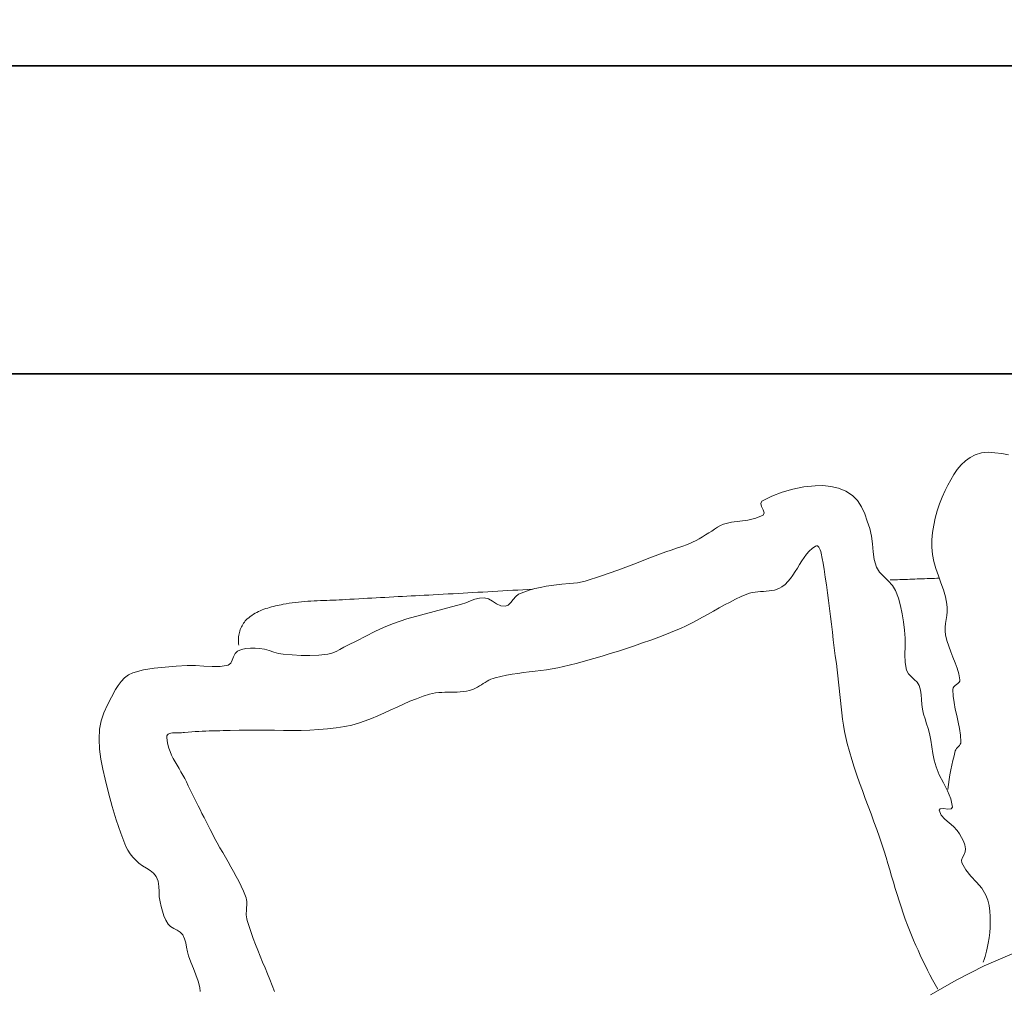
# Model space of a CAD drawing. Units: inches. Extents: x -36302355 to 648, y -221479757 to 75.
# Tile 34 of 37: x 283 to 311, y -2 to 26. Entities that reach past the tile are written whole.
import ezdxf

# ---------------------------------------------------------------- set-up
doc = ezdxf.new("R2010")
doc.units = ezdxf.units.IN
doc.header["$MEASUREMENT"] = 0
for name, color, linetype, lineweight in [('A-ANNO-DIMS', 2, 'Continuous', 18), ('A-FURN', 8, 'Continuous', 13), ('A-WALL', 7, 'Continuous', 35)]:
    doc.layers.add(name, color=color, linetype=linetype, lineweight=lineweight)
doc.styles.get("Standard").update_dxf_attribs({"font": 'arial.ttf'})
doc.dimstyles.get("Standard").update_dxf_attribs({"dimtxt": 0.18, "dimasz": 0.18, "dimexe": 0.18, "dimexo": 0.0625, "dimgap": 0.09, "dimtad": 0, "dimtih": 1, "dimtoh": 1, "dimdec": 0, "dimzin": 0, "dimdsep": 46, "dimlunit": 3, "dimtxsty": 'Standard', "dimcen": 0.09, "dimadec": 0, "dimazin": 0, "dimtfac": 1, "dimtdec": 0, "dimtofl": 0, "dimtmove": 0, "dimatfit": 3, "dimfxl": 1, "dimtolj": 1, "dimtzin": 0, "dimarcsym": 0})

# ---------------------------------------------------------------- blocks, each defined once
blk = doc.blocks.new('*D4')
at = {"layer": 'A-ANNO-DIMS', "color": 0, "lineweight": -2, "transparency": 16777216}
for p, q in [((145.197, 25.043), (145.197, 71.11)), ((605.197, 25.043), (605.197, 71.11)), ((145.377, 70.93), (364.803, 70.93)), ((605.017, 70.93), (385.59, 70.93))]:
    blk.add_line(p, q, dxfattribs=at)
at = {"layer": 'A-ANNO-DIMS', "color": 0, "transparency": 16777216}
for points in [[(145.377, 70.96), (145.377, 70.9), (145.197, 70.93)], [(605.017, 70.96), (605.017, 70.9), (605.197, 70.93)]]:
    blk.add_solid(points, dxfattribs=at)
at = {"layer": 'Defpoints', "color": 0, "transparency": 16777216}
for p in [(605.197, 70.93), (145.197, 24.981), (605.197, 24.981)]:
    blk.add_point(p, dxfattribs=at)
at = {"layer": 'A-ANNO-DIMS', "color": 0, "transparency": 16777216, "insert": (375.197, 70.93), "char_height": 6, "attachment_point": 5}
blk.add_mtext('\\A1;38\'-4"', dxfattribs=at)
blk = doc.blocks.new('BED-DOUBLE')
for p, q in [((26.943, 79.401), (26.757, 79.348)), ((27.135, 79.418), (26.943, 79.401)), ((27.332, 79.407), (27.135, 79.418)), ((27.532, 79.381), (27.332, 79.407)), ((27.733, 79.348), (27.532, 79.381)), ((26.471, 79.169), (26.347, 79.049)), ((26.607, 79.27), (26.471, 79.169)), ((26.757, 79.348), (26.607, 79.27)), ((26.235, 78.914), (26.134, 78.768)), ((26.347, 79.049), (26.235, 78.914)), ((26.042, 78.615), (25.959, 78.459)), ((26.134, 78.768), (26.042, 78.615)), ((20.815, 78.133), (21.12, 78.252)), ((21.12, 78.252), (21.435, 78.344)), ((21.435, 78.344), (21.756, 78.407)), ((21.756, 78.407), (22.08, 78.443)), ((22.08, 78.443), (22.309, 78.445)), ((22.309, 78.445), (22.541, 78.42)), ((22.541, 78.42), (22.768, 78.366)), ((22.768, 78.366), (22.981, 78.28)), ((22.981, 78.28), (23.172, 78.159)), ((25.883, 78.303), (25.797, 78.108)), ((25.959, 78.459), (25.883, 78.303)), ((20.495, 77.926), (20.524, 77.986)), ((20.521, 77.836), (20.495, 77.926)), ((20.524, 77.986), (20.815, 78.133)), ((23.172, 78.159), (23.323, 78.006)), ((23.323, 78.006), (23.44, 77.822)), ((25.797, 78.108), (25.719, 77.908)), ((20.567, 77.736), (20.521, 77.836)), ((20.565, 77.584), (20.594, 77.646)), ((20.594, 77.646), (20.567, 77.736)), ((23.44, 77.822), (23.532, 77.618)), ((25.65, 77.704), (25.593, 77.496)), ((25.719, 77.908), (25.65, 77.704)), ((19.408, 77.323), (19.64, 77.378)), ((19.64, 77.378), (19.88, 77.41)), ((19.88, 77.41), (20.119, 77.44)), ((20.119, 77.44), (20.35, 77.491)), ((20.35, 77.491), (20.565, 77.584)), ((23.532, 77.618), (23.607, 77.405)), ((23.607, 77.405), (23.677, 77.194)), ((25.593, 77.496), (25.546, 77.286)), ((18.887, 77.007), (18.98, 77.065)), ((18.98, 77.065), (19.065, 77.119)), ((19.065, 77.119), (19.147, 77.177)), ((19.147, 77.177), (19.23, 77.234)), ((19.23, 77.234), (19.317, 77.284)), ((19.317, 77.284), (19.408, 77.323)), ((23.677, 77.194), (23.73, 76.972)), ((25.513, 77.074), (25.494, 76.862)), ((25.546, 77.286), (25.513, 77.074)), ((18.352, 76.726), (18.506, 76.789)), ((18.506, 76.789), (18.605, 76.837)), ((18.605, 76.837), (18.7, 76.891)), ((18.7, 76.891), (18.794, 76.949)), ((18.794, 76.949), (18.887, 77.007)), ((23.73, 76.972), (23.756, 76.743)), ((25.494, 76.862), (25.489, 76.649)), ((17.253, 76.332), (17.722, 76.507)), ((17.722, 76.507), (17.88, 76.561)), ((17.88, 76.561), (18.038, 76.614)), ((18.038, 76.614), (18.196, 76.668)), ((18.196, 76.668), (18.352, 76.726)), ((21.833, 76.44), (21.911, 76.527)), ((21.911, 76.527), (21.997, 76.607)), ((21.997, 76.607), (22.092, 76.675)), ((22.092, 76.675), (22.122, 76.687)), ((22.122, 76.687), (22.15, 76.685)), ((22.15, 76.685), (22.174, 76.67)), ((22.174, 76.67), (22.196, 76.645)), ((22.196, 76.645), (22.215, 76.61)), ((22.215, 76.61), (22.232, 76.569)), ((22.232, 76.569), (22.247, 76.522)), ((22.247, 76.522), (22.26, 76.472)), ((23.756, 76.743), (23.776, 76.512)), ((23.776, 76.512), (23.809, 76.285)), ((25.489, 76.649), (25.507, 76.436)), ((16.786, 76.152), (17.253, 76.332)), ((21.628, 76.142), (21.693, 76.245)), ((21.693, 76.245), (21.761, 76.345)), ((21.761, 76.345), (21.833, 76.44)), ((22.26, 76.472), (22.271, 76.419)), ((22.271, 76.419), (22.281, 76.367)), ((22.281, 76.367), (22.29, 76.317)), ((22.29, 76.317), (22.297, 76.271)), ((22.297, 76.271), (22.304, 76.23)), ((22.304, 76.23), (22.343, 76.002)), ((23.809, 76.285), (23.875, 76.067)), ((25.507, 76.436), (25.55, 76.227)), ((25.55, 76.227), (25.61, 76.02)), ((15.847, 75.807), (16.318, 75.975)), ((16.318, 75.975), (16.786, 76.152)), ((21.434, 75.833), (21.5, 75.934)), ((21.5, 75.934), (21.565, 76.038)), ((21.565, 76.038), (21.628, 76.142)), ((22.343, 76.002), (22.38, 75.774)), ((23.875, 76.067), (23.965, 75.917)), ((23.965, 75.917), (24.086, 75.786)), ((25.61, 76.02), (25.681, 75.814)), ((15.145, 75.609), (15.37, 75.658)), ((15.37, 75.658), (15.847, 75.807)), ((21.205, 75.561), (21.288, 75.644)), ((21.288, 75.644), (21.364, 75.736)), ((21.364, 75.736), (21.434, 75.833)), ((22.38, 75.774), (22.414, 75.545)), ((24.086, 75.786), (24.218, 75.662)), ((24.218, 75.662), (24.341, 75.531)), ((24.272, 75.689), (24.344, 75.691)), ((24.344, 75.691), (24.416, 75.694)), ((24.416, 75.694), (24.488, 75.697)), ((24.488, 75.697), (24.56, 75.699)), ((24.56, 75.699), (24.632, 75.702)), ((24.632, 75.702), (24.704, 75.704)), ((24.704, 75.704), (24.776, 75.707)), ((24.776, 75.707), (24.848, 75.709)), ((24.848, 75.709), (24.92, 75.712)), ((24.92, 75.712), (24.992, 75.714)), ((24.992, 75.714), (25.064, 75.717)), ((25.064, 75.717), (25.136, 75.719)), ((25.136, 75.719), (25.208, 75.722)), ((25.208, 75.722), (25.28, 75.724)), ((25.28, 75.724), (25.353, 75.727)), ((25.353, 75.727), (25.425, 75.729)), ((25.425, 75.729), (25.497, 75.732)), ((25.497, 75.732), (25.569, 75.734)), ((25.569, 75.734), (25.641, 75.737)), ((25.641, 75.737), (25.713, 75.74)), ((25.681, 75.814), (25.756, 75.609)), ((12.093, 75.321), (12.238, 75.329)), ((12.238, 75.329), (12.384, 75.337)), ((12.384, 75.337), (12.53, 75.345)), ((12.53, 75.345), (12.675, 75.353)), ((12.675, 75.353), (12.821, 75.362)), ((12.821, 75.362), (12.966, 75.37)), ((12.966, 75.37), (13.112, 75.378)), ((13.112, 75.378), (13.258, 75.386)), ((13.258, 75.386), (13.403, 75.395)), ((13.403, 75.395), (13.549, 75.403)), ((13.425, 75.27), (13.578, 75.336)), ((13.549, 75.403), (13.694, 75.411)), ((13.578, 75.336), (13.736, 75.39)), ((13.694, 75.411), (13.84, 75.419)), ((13.736, 75.39), (13.898, 75.435)), ((13.898, 75.435), (14.062, 75.473)), ((14.062, 75.473), (14.226, 75.506)), ((14.226, 75.506), (14.454, 75.541)), ((14.454, 75.541), (14.685, 75.562)), ((14.685, 75.562), (14.916, 75.581)), ((14.916, 75.581), (15.145, 75.609)), ((20.248, 75.322), (20.328, 75.335)), ((20.328, 75.335), (20.41, 75.344)), ((20.41, 75.344), (20.493, 75.35)), ((20.493, 75.35), (20.576, 75.355)), ((20.576, 75.355), (20.658, 75.36)), ((20.658, 75.36), (20.74, 75.367)), ((20.74, 75.367), (20.82, 75.378)), ((20.82, 75.378), (20.898, 75.394)), ((20.898, 75.394), (20.973, 75.417)), ((20.973, 75.417), (21.045, 75.447)), ((21.045, 75.447), (21.112, 75.488)), ((21.112, 75.488), (21.205, 75.561)), ((22.414, 75.545), (22.446, 75.315)), ((24.341, 75.531), (24.434, 75.383)), ((24.434, 75.383), (24.518, 75.161)), ((25.756, 75.609), (25.827, 75.404)), ((25.827, 75.404), (25.889, 75.196)), ((6.907, 75.034), (6.998, 75.044)), ((6.998, 75.044), (7.089, 75.053)), ((7.089, 75.053), (7.18, 75.06)), ((7.18, 75.06), (7.272, 75.067)), ((7.272, 75.067), (7.363, 75.072)), ((7.363, 75.072), (7.455, 75.077)), ((7.455, 75.077), (7.547, 75.081)), ((7.547, 75.081), (7.639, 75.085)), ((7.639, 75.085), (7.73, 75.088)), ((7.73, 75.088), (7.822, 75.091)), ((7.822, 75.091), (7.914, 75.095)), ((7.914, 75.095), (8.006, 75.098)), ((8.006, 75.098), (8.098, 75.102)), ((8.098, 75.102), (8.189, 75.106)), ((8.189, 75.106), (8.281, 75.11)), ((8.281, 75.11), (8.372, 75.116)), ((8.372, 75.116), (8.5, 75.124)), ((8.5, 75.124), (8.628, 75.131)), ((8.628, 75.131), (8.756, 75.139)), ((8.756, 75.139), (8.883, 75.146)), ((8.883, 75.146), (9.011, 75.154)), ((9.011, 75.154), (9.139, 75.161)), ((9.139, 75.161), (9.267, 75.168)), ((9.267, 75.168), (9.394, 75.175)), ((9.394, 75.175), (9.522, 75.181)), ((9.522, 75.181), (9.65, 75.188)), ((9.65, 75.188), (9.778, 75.195)), ((9.778, 75.195), (9.906, 75.201)), ((9.906, 75.201), (10.033, 75.208)), ((10.033, 75.208), (10.161, 75.215)), ((10.161, 75.215), (10.289, 75.221)), ((10.289, 75.221), (10.417, 75.228)), ((10.417, 75.228), (10.545, 75.235)), ((10.545, 75.235), (10.672, 75.242)), ((10.672, 75.242), (10.8, 75.248)), ((10.8, 75.248), (10.928, 75.255)), ((10.928, 75.255), (11.074, 75.264)), ((11.074, 75.264), (11.219, 75.272)), ((11.219, 75.272), (11.365, 75.28)), ((11.365, 75.28), (11.511, 75.288)), ((11.511, 75.288), (11.656, 75.296)), ((11.656, 75.296), (11.802, 75.304)), ((11.802, 75.304), (11.947, 75.312)), ((11.888, 75.025), (12.019, 75.077)), ((11.947, 75.312), (12.093, 75.321)), ((12.019, 75.077), (12.151, 75.125)), ((12.151, 75.125), (12.284, 75.159)), ((12.284, 75.159), (12.419, 75.168)), ((12.419, 75.168), (12.546, 75.136)), ((12.546, 75.136), (12.666, 75.069)), ((12.666, 75.069), (12.784, 74.994)), ((13.199, 75.028), (13.268, 75.118)), ((13.268, 75.118), (13.34, 75.205)), ((13.34, 75.205), (13.425, 75.27)), ((19.437, 74.959), (19.599, 75.045)), ((19.599, 75.045), (19.762, 75.127)), ((19.762, 75.127), (19.927, 75.205)), ((19.927, 75.205), (20.094, 75.277)), ((20.094, 75.277), (20.17, 75.303)), ((20.17, 75.303), (20.248, 75.322)), ((22.446, 75.315), (22.476, 75.086)), ((22.476, 75.086), (22.505, 74.856)), ((24.518, 75.161), (24.58, 74.932)), ((25.889, 75.196), (25.933, 74.985)), ((5.779, 74.741), (5.83, 74.766)), ((5.83, 74.766), (5.882, 74.79)), ((5.882, 74.79), (5.935, 74.812)), ((5.935, 74.812), (5.988, 74.832)), ((5.988, 74.832), (6.043, 74.852)), ((6.043, 74.852), (6.098, 74.869)), ((6.098, 74.869), (6.153, 74.886)), ((6.153, 74.886), (6.209, 74.902)), ((6.209, 74.902), (6.265, 74.916)), ((6.265, 74.916), (6.322, 74.93)), ((6.322, 74.93), (6.378, 74.943)), ((6.378, 74.943), (6.434, 74.955)), ((6.434, 74.955), (6.49, 74.967)), ((6.49, 74.967), (6.546, 74.978)), ((6.546, 74.978), (6.636, 74.995)), ((6.636, 74.995), (6.726, 75.01)), ((6.726, 75.01), (6.816, 75.023)), ((6.816, 75.023), (6.907, 75.034)), ((10.558, 74.665), (10.958, 74.77)), ((10.958, 74.77), (11.358, 74.873)), ((11.358, 74.873), (11.757, 74.981)), ((11.757, 74.981), (11.888, 75.025)), ((12.784, 74.994), (12.904, 74.935)), ((12.904, 74.935), (13.03, 74.919)), ((13.03, 74.919), (13.123, 74.955)), ((13.123, 74.955), (13.199, 75.028)), ((18.958, 74.692), (19.118, 74.782)), ((19.118, 74.782), (19.277, 74.871)), ((19.277, 74.871), (19.437, 74.959)), ((22.505, 74.856), (22.533, 74.626)), ((24.58, 74.932), (24.626, 74.698)), ((25.939, 74.761), (25.927, 74.648)), ((25.933, 74.985), (25.942, 74.873)), ((25.942, 74.873), (25.939, 74.761)), ((5.419, 74.459), (5.445, 74.491)), ((5.445, 74.491), (5.472, 74.521)), ((5.472, 74.521), (5.501, 74.549)), ((5.501, 74.549), (5.544, 74.587)), ((5.544, 74.587), (5.588, 74.622)), ((5.588, 74.622), (5.633, 74.654)), ((5.633, 74.654), (5.68, 74.685)), ((5.68, 74.685), (5.729, 74.714)), ((5.729, 74.714), (5.779, 74.741)), ((9.77, 74.421), (10.161, 74.551)), ((10.161, 74.551), (10.558, 74.665)), ((18.476, 74.431), (18.638, 74.516)), ((18.638, 74.516), (18.798, 74.603)), ((18.798, 74.603), (18.958, 74.692)), ((22.533, 74.626), (22.56, 74.396)), ((24.626, 74.698), (24.663, 74.462)), ((25.911, 74.534), (25.895, 74.421)), ((25.927, 74.648), (25.911, 74.534)), ((5.273, 74.156), (5.285, 74.197)), ((5.285, 74.197), (5.299, 74.237)), ((5.299, 74.237), (5.314, 74.277)), ((5.314, 74.277), (5.332, 74.316)), ((5.332, 74.316), (5.351, 74.353)), ((5.351, 74.353), (5.372, 74.39)), ((5.372, 74.39), (5.395, 74.425)), ((5.395, 74.425), (5.419, 74.459)), ((8.965, 74.05), (9.228, 74.184)), ((9.228, 74.184), (9.496, 74.31)), ((9.496, 74.31), (9.77, 74.421)), ((17.748, 74.11), (17.98, 74.202)), ((17.98, 74.202), (18.148, 74.273)), ((18.148, 74.273), (18.313, 74.35)), ((18.313, 74.35), (18.476, 74.431)), ((22.56, 74.396), (22.588, 74.166)), ((24.663, 74.462), (24.695, 74.226)), ((24.695, 74.226), (24.712, 73.99)), ((25.884, 74.308), (25.882, 74.196)), ((25.882, 74.196), (25.893, 74.084)), ((25.895, 74.421), (25.884, 74.308)), ((5.242, 73.946), (5.244, 73.988)), ((5.242, 73.905), (5.242, 73.946)), ((5.245, 73.864), (5.242, 73.905)), ((5.244, 73.988), (5.248, 74.03)), ((5.248, 74.03), (5.254, 74.072)), ((5.254, 74.072), (5.262, 74.114)), ((5.262, 74.114), (5.273, 74.156)), ((8.436, 73.783), (8.701, 73.914)), ((8.701, 73.914), (8.965, 74.05)), ((17.047, 73.851), (17.282, 73.935)), ((17.282, 73.935), (17.515, 74.022)), ((17.515, 74.022), (17.748, 74.11)), ((22.588, 74.166), (22.615, 73.936)), ((22.615, 73.936), (22.643, 73.706)), ((24.712, 73.99), (24.71, 73.753)), ((25.893, 74.084), (25.931, 73.917)), ((25.931, 73.917), (25.983, 73.753)), ((5.146, 73.544), (5.214, 73.612)), ((5.214, 73.612), (5.335, 73.661)), ((5.249, 73.823), (5.245, 73.864)), ((5.256, 73.784), (5.249, 73.823)), ((5.335, 73.661), (5.463, 73.688)), ((5.463, 73.688), (5.596, 73.698)), ((5.596, 73.698), (5.731, 73.697)), ((5.731, 73.697), (5.863, 73.69)), ((5.863, 73.69), (6.003, 73.668)), ((6.003, 73.668), (6.139, 73.629)), ((6.139, 73.629), (6.275, 73.584)), ((8.094, 73.6), (8.208, 73.66)), ((8.208, 73.66), (8.321, 73.724)), ((8.321, 73.724), (8.436, 73.783)), ((16.101, 73.538), (16.338, 73.612)), ((16.338, 73.612), (16.575, 73.69)), ((16.575, 73.69), (16.812, 73.769)), ((16.812, 73.769), (17.047, 73.851)), ((22.643, 73.706), (22.672, 73.476)), ((24.71, 73.753), (24.706, 73.515)), ((25.983, 73.753), (26.044, 73.592)), ((5.019, 73.255), (5.066, 73.344)), ((5.066, 73.344), (5.102, 73.448)), ((5.102, 73.448), (5.146, 73.544)), ((6.275, 73.584), (6.411, 73.544)), ((6.411, 73.544), (6.55, 73.52)), ((6.55, 73.52), (6.81, 73.5)), ((6.81, 73.5), (7.072, 73.487)), ((7.072, 73.487), (7.333, 73.484)), ((7.333, 73.484), (7.594, 73.494)), ((7.594, 73.494), (7.853, 73.521)), ((7.853, 73.521), (7.976, 73.551)), ((7.976, 73.551), (8.094, 73.6)), ((15.143, 73.26), (15.383, 73.326)), ((15.383, 73.326), (15.623, 73.395)), ((15.623, 73.395), (15.862, 73.465)), ((15.862, 73.465), (16.101, 73.538)), ((22.672, 73.476), (22.703, 73.247)), ((24.706, 73.515), (24.715, 73.279)), ((26.044, 73.592), (26.109, 73.431)), ((26.109, 73.431), (26.174, 73.271)), ((2.158, 72.979), (2.468, 73.062)), ((2.468, 73.062), (2.784, 73.114)), ((2.784, 73.114), (3.106, 73.145)), ((3.106, 73.145), (3.429, 73.167)), ((3.429, 73.167), (3.751, 73.188)), ((3.751, 73.188), (3.991, 73.191)), ((3.991, 73.191), (4.232, 73.175)), ((4.232, 73.175), (4.474, 73.159)), ((4.474, 73.159), (4.712, 73.161)), ((4.712, 73.161), (4.945, 73.202)), ((4.945, 73.202), (5.019, 73.255)), ((13.905, 73.023), (14.073, 73.045)), ((14.073, 73.045), (14.24, 73.068)), ((14.24, 73.068), (14.407, 73.094)), ((14.407, 73.094), (14.573, 73.123)), ((14.573, 73.123), (14.738, 73.157)), ((14.738, 73.157), (14.902, 73.196)), ((14.902, 73.196), (15.143, 73.26)), ((22.703, 73.247), (22.726, 73.067)), ((22.726, 73.067), (22.746, 72.887)), ((24.715, 73.279), (24.755, 73.049)), ((24.755, 73.049), (24.805, 72.949)), ((26.174, 73.271), (26.233, 73.109)), ((26.233, 73.109), (26.28, 72.944)), ((1.822, 72.725), (1.921, 72.832)), ((1.921, 72.832), (2.033, 72.919)), ((2.033, 72.919), (2.158, 72.979)), ((12.504, 72.732), (12.56, 72.763)), ((12.56, 72.763), (12.619, 72.791)), ((12.619, 72.791), (12.678, 72.815)), ((12.678, 72.815), (12.74, 72.833)), ((12.74, 72.833), (12.904, 72.872)), ((12.904, 72.872), (13.069, 72.905)), ((13.069, 72.905), (13.235, 72.933)), ((13.235, 72.933), (13.402, 72.958)), ((13.402, 72.958), (13.57, 72.981)), ((13.57, 72.981), (13.738, 73.003)), ((13.738, 73.003), (13.905, 73.023)), ((22.746, 72.887), (22.765, 72.706)), ((24.805, 72.949), (24.884, 72.864)), ((24.884, 72.864), (24.976, 72.786)), ((24.976, 72.786), (25.061, 72.704)), ((26.28, 72.944), (26.312, 72.776)), ((26.312, 72.776), (26.308, 72.735)), ((1.534, 72.267), (1.658, 72.486)), ((1.658, 72.486), (1.735, 72.608)), ((1.735, 72.608), (1.822, 72.725)), ((11.901, 72.44), (11.989, 72.458)), ((11.989, 72.458), (12.05, 72.477)), ((12.05, 72.477), (12.11, 72.501)), ((12.11, 72.501), (12.168, 72.529)), ((12.168, 72.529), (12.225, 72.56)), ((12.225, 72.56), (12.281, 72.593)), ((12.281, 72.593), (12.337, 72.628)), ((12.337, 72.628), (12.392, 72.663)), ((12.392, 72.663), (12.448, 72.698)), ((12.448, 72.698), (12.504, 72.732)), ((22.765, 72.706), (22.784, 72.525)), ((22.784, 72.525), (22.802, 72.344)), ((25.061, 72.704), (25.122, 72.608)), ((25.122, 72.608), (25.161, 72.474)), ((25.161, 72.474), (25.18, 72.335)), ((26.111, 72.533), (26.102, 72.492)), ((26.102, 72.492), (26.114, 72.299)), ((26.136, 72.57), (26.111, 72.533)), ((26.172, 72.603), (26.136, 72.57)), ((26.212, 72.634), (26.172, 72.603)), ((26.252, 72.666), (26.212, 72.634)), ((26.286, 72.699), (26.252, 72.666)), ((26.308, 72.735), (26.286, 72.699)), ((1.417, 72.042), (1.534, 72.267)), ((10.253, 72.144), (10.442, 72.221)), ((10.442, 72.221), (10.634, 72.291)), ((10.634, 72.291), (10.828, 72.353)), ((10.828, 72.353), (10.915, 72.374)), ((10.915, 72.374), (11.003, 72.389)), ((11.003, 72.389), (11.092, 72.399)), ((11.092, 72.399), (11.181, 72.406)), ((11.181, 72.406), (11.271, 72.409)), ((11.271, 72.409), (11.362, 72.41)), ((11.362, 72.41), (11.453, 72.411)), ((11.453, 72.411), (11.543, 72.412)), ((11.543, 72.412), (11.634, 72.414)), ((11.634, 72.414), (11.723, 72.419)), ((11.723, 72.419), (11.813, 72.427)), ((11.813, 72.427), (11.901, 72.44)), ((22.802, 72.344), (22.82, 72.164)), ((22.82, 72.164), (22.84, 71.983)), ((25.18, 72.335), (25.188, 72.193)), ((25.188, 72.193), (25.197, 72.051)), ((26.114, 72.299), (26.14, 72.108)), ((1.316, 71.81), (1.417, 72.042)), ((9.506, 71.805), (9.692, 71.891)), ((9.692, 71.891), (9.878, 71.977)), ((9.878, 71.977), (10.065, 72.062)), ((10.065, 72.062), (10.253, 72.144)), ((22.84, 71.983), (22.862, 71.803)), ((25.197, 72.051), (25.217, 71.912)), ((25.217, 71.912), (25.252, 71.769)), ((26.14, 72.108), (26.176, 71.917)), ((26.176, 71.917), (26.217, 71.727)), ((1.238, 71.572), (1.316, 71.81)), ((8.94, 71.57), (9.13, 71.643)), ((9.13, 71.643), (9.318, 71.722)), ((9.318, 71.722), (9.506, 71.805)), ((22.862, 71.803), (22.886, 71.623)), ((22.886, 71.623), (22.914, 71.444)), ((25.252, 71.769), (25.294, 71.628)), ((25.294, 71.628), (25.339, 71.487)), ((26.217, 71.727), (26.258, 71.537)), ((1.175, 71.036), (1.19, 71.327)), ((1.19, 71.327), (1.238, 71.572)), ((5.007, 71.296), (5.264, 71.303)), ((5.264, 71.303), (5.523, 71.305)), ((5.523, 71.305), (5.781, 71.304)), ((5.781, 71.304), (6.04, 71.301)), ((7.074, 71.296), (7.332, 71.303)), ((7.332, 71.303), (7.589, 71.317)), ((7.589, 71.317), (7.845, 71.338)), ((7.845, 71.338), (8.1, 71.368)), ((8.1, 71.368), (8.354, 71.408)), ((8.354, 71.408), (8.553, 71.451)), ((8.553, 71.451), (8.748, 71.506)), ((8.748, 71.506), (8.94, 71.57)), ((22.914, 71.444), (22.945, 71.266)), ((25.339, 71.487), (25.382, 71.346)), ((25.382, 71.346), (25.42, 71.204)), ((26.258, 71.537), (26.296, 71.346)), ((26.296, 71.346), (26.325, 71.155)), ((1.191, 70.743), (1.175, 71.036)), ((3.15, 71.095), (3.155, 71.133)), ((3.16, 70.987), (3.15, 71.095)), ((3.155, 71.133), (3.171, 71.163)), ((3.171, 71.163), (3.197, 71.186)), ((3.197, 71.186), (3.231, 71.202)), ((3.231, 71.202), (3.271, 71.214)), ((3.271, 71.214), (3.318, 71.222)), ((3.318, 71.222), (3.368, 71.226)), ((3.368, 71.226), (3.421, 71.228)), ((3.421, 71.228), (3.475, 71.228)), ((3.475, 71.228), (3.529, 71.228)), ((3.529, 71.228), (3.581, 71.228)), ((3.581, 71.228), (3.63, 71.229)), ((3.63, 71.229), (3.674, 71.232)), ((3.674, 71.232), (3.776, 71.243)), ((3.776, 71.243), (3.879, 71.251)), ((3.879, 71.251), (3.981, 71.258)), ((3.981, 71.258), (4.083, 71.264)), ((4.083, 71.264), (4.186, 71.27)), ((4.186, 71.27), (4.288, 71.274)), ((4.288, 71.274), (4.391, 71.277)), ((4.391, 71.277), (4.494, 71.281)), ((4.494, 71.281), (4.596, 71.283)), ((4.596, 71.283), (4.699, 71.286)), ((4.699, 71.286), (4.801, 71.289)), ((4.801, 71.289), (4.904, 71.292)), ((4.904, 71.292), (5.007, 71.296)), ((6.04, 71.301), (6.299, 71.297)), ((6.299, 71.297), (6.558, 71.294)), ((6.558, 71.294), (6.816, 71.293)), ((6.816, 71.293), (7.074, 71.296)), ((22.945, 71.266), (22.982, 71.089)), ((22.982, 71.089), (23.023, 70.912)), ((25.42, 71.204), (25.46, 71.009)), ((26.325, 71.155), (26.341, 70.962)), ((1.231, 70.451), (1.191, 70.743)), ((3.18, 70.881), (3.16, 70.987)), ((3.21, 70.777), (3.18, 70.881)), ((3.248, 70.675), (3.21, 70.777)), ((23.023, 70.912), (23.085, 70.679)), ((25.46, 71.009), (25.493, 70.813)), ((25.493, 70.813), (25.525, 70.617)), ((26.192, 70.731), (26.177, 70.695)), ((26.215, 70.764), (26.192, 70.731)), ((26.242, 70.796), (26.215, 70.764)), ((26.271, 70.827), (26.242, 70.796)), ((26.298, 70.858), (26.271, 70.827)), ((26.321, 70.891), (26.298, 70.858)), ((26.336, 70.925), (26.321, 70.891)), ((26.341, 70.962), (26.336, 70.925)), ((1.287, 70.16), (1.231, 70.451)), ((3.292, 70.575), (3.248, 70.675)), ((3.341, 70.476), (3.292, 70.575)), ((3.395, 70.377), (3.341, 70.476)), ((23.085, 70.679), (23.153, 70.448)), ((23.153, 70.448), (23.225, 70.218)), ((25.525, 70.617), (25.564, 70.423)), ((26.14, 70.556), (26.106, 70.417)), ((26.177, 70.695), (26.14, 70.556)), ((1.35, 69.873), (1.287, 70.16)), ((3.451, 70.28), (3.395, 70.377)), ((3.509, 70.182), (3.451, 70.28)), ((3.566, 70.085), (3.509, 70.182)), ((23.225, 70.218), (23.302, 69.989)), ((25.564, 70.423), (25.614, 70.231)), ((25.614, 70.231), (25.71, 69.993)), ((26.074, 70.278), (26.045, 70.138)), ((26.106, 70.417), (26.074, 70.278)), ((1.446, 69.472), (1.35, 69.873)), ((3.622, 69.988), (3.566, 70.085)), ((3.676, 69.89), (3.622, 69.988)), ((3.725, 69.791), (3.676, 69.89)), ((23.302, 69.989), (23.381, 69.761)), ((25.71, 69.993), (25.829, 69.762)), ((26.019, 69.997), (25.995, 69.856)), ((26.045, 70.138), (26.019, 69.997)), ((3.78, 69.675), (3.725, 69.791)), ((3.836, 69.558), (3.78, 69.675)), ((23.381, 69.761), (23.463, 69.534)), ((25.829, 69.762), (25.948, 69.531)), ((25.974, 69.714), (25.956, 69.572)), ((25.995, 69.856), (25.974, 69.714)), ((1.554, 69.073), (1.446, 69.472)), ((3.893, 69.442), (3.836, 69.558)), ((3.949, 69.326), (3.893, 69.442)), ((4.007, 69.21), (3.949, 69.326)), ((23.463, 69.534), (23.547, 69.307)), ((23.547, 69.307), (23.632, 69.08)), ((25.948, 69.531), (26.043, 69.295)), ((26.043, 69.295), (26.093, 69.048)), ((1.675, 68.678), (1.554, 69.073)), ((4.064, 69.095), (4.007, 69.21)), ((4.122, 68.979), (4.064, 69.095)), ((23.632, 69.08), (23.716, 68.854)), ((25.738, 69.008), (25.707, 68.962)), ((25.834, 69.01), (25.738, 69.008)), ((25.954, 68.998), (25.834, 69.01)), ((26.054, 69.001), (25.954, 68.998)), ((26.093, 69.048), (26.054, 69.001)), ((4.18, 68.864), (4.122, 68.979)), ((4.239, 68.749), (4.18, 68.864)), ((4.298, 68.634), (4.239, 68.749)), ((23.716, 68.854), (23.801, 68.627)), ((25.707, 68.962), (25.768, 68.822)), ((25.768, 68.822), (25.873, 68.704)), ((1.809, 68.288), (1.675, 68.678)), ((4.357, 68.519), (4.298, 68.634)), ((4.416, 68.404), (4.357, 68.519)), ((23.801, 68.627), (23.883, 68.4)), ((25.873, 68.704), (25.999, 68.598)), ((25.999, 68.598), (26.127, 68.49)), ((26.127, 68.49), (26.234, 68.369)), ((1.956, 67.902), (1.809, 68.288)), ((4.475, 68.289), (4.416, 68.404)), ((4.55, 68.148), (4.475, 68.289)), ((4.627, 68.007), (4.55, 68.148)), ((23.883, 68.4), (23.964, 68.172)), ((23.964, 68.172), (24.041, 67.944)), ((26.234, 68.369), (26.299, 68.27)), ((26.299, 68.27), (26.36, 68.166)), ((26.36, 68.166), (26.413, 68.059)), ((2.012, 67.792), (1.956, 67.902)), ((4.705, 67.868), (4.627, 68.007)), ((4.785, 67.729), (4.705, 67.868)), ((24.041, 67.944), (24.1, 67.764)), ((26.413, 68.059), (26.454, 67.948)), ((26.454, 67.948), (26.479, 67.833)), ((2.082, 67.69), (2.012, 67.792)), ((2.164, 67.594), (2.082, 67.69)), ((2.251, 67.503), (2.164, 67.594)), ((4.865, 67.59), (4.785, 67.729)), ((4.945, 67.451), (4.865, 67.59)), ((24.1, 67.764), (24.156, 67.584)), ((24.156, 67.584), (24.211, 67.403)), ((26.386, 67.585), (26.357, 67.505)), ((26.431, 67.667), (26.386, 67.585)), ((26.469, 67.749), (26.431, 67.667)), ((26.479, 67.833), (26.469, 67.749)), ((2.34, 67.415), (2.251, 67.503)), ((2.441, 67.335), (2.34, 67.415)), ((2.555, 67.267), (2.441, 67.335)), ((5.025, 67.311), (4.945, 67.451)), ((5.102, 67.171), (5.025, 67.311)), ((24.211, 67.403), (24.264, 67.222)), ((26.357, 67.505), (26.365, 67.427)), ((26.365, 67.427), (26.483, 67.224)), ((2.668, 67.2), (2.555, 67.267)), ((2.769, 67.123), (2.668, 67.2)), ((2.846, 67.024), (2.769, 67.123)), ((2.898, 66.886), (2.846, 67.024)), ((5.178, 67.03), (5.102, 67.171)), ((5.252, 66.888), (5.178, 67.03)), ((24.264, 67.222), (24.318, 67.041)), ((24.318, 67.041), (24.371, 66.86)), ((26.483, 67.224), (26.632, 67.041)), ((26.632, 67.041), (26.794, 66.864)), ((2.92, 66.738), (2.898, 66.886)), ((2.927, 66.585), (2.92, 66.738)), ((5.322, 66.745), (5.252, 66.888)), ((5.388, 66.599), (5.322, 66.745)), ((24.371, 66.86), (24.424, 66.679)), ((26.794, 66.864), (26.947, 66.682)), ((2.934, 66.432), (2.927, 66.585)), ((2.957, 66.283), (2.934, 66.432)), ((5.45, 66.452), (5.388, 66.599)), ((5.467, 66.4), (5.45, 66.452)), ((24.424, 66.679), (24.479, 66.498)), ((24.479, 66.498), (24.534, 66.317)), ((26.947, 66.682), (27.07, 66.482)), ((27.07, 66.482), (27.127, 66.334)), ((2.99, 66.148), (2.957, 66.283)), ((3.026, 66.014), (2.99, 66.148)), ((5.478, 66.347), (5.467, 66.4)), ((5.485, 66.293), (5.478, 66.347)), ((5.48, 66.07), (5.483, 66.126)), ((5.483, 66.126), (5.486, 66.183)), ((5.487, 66.238), (5.485, 66.293)), ((5.486, 66.183), (5.487, 66.238)), ((24.534, 66.317), (24.592, 66.138)), ((24.592, 66.138), (24.652, 65.959)), ((27.127, 66.334), (27.163, 66.178)), ((27.163, 66.178), (27.184, 66.017)), ((3.068, 65.882), (3.026, 66.014)), ((3.122, 65.755), (3.068, 65.882)), ((5.474, 65.958), (5.476, 66.014)), ((5.474, 65.902), (5.474, 65.958)), ((5.478, 65.847), (5.474, 65.902)), ((5.476, 66.014), (5.48, 66.07)), ((5.486, 65.793), (5.478, 65.847)), ((24.652, 65.959), (24.715, 65.781)), ((27.184, 66.017), (27.194, 65.855)), ((27.194, 65.855), (27.198, 65.694)), ((3.19, 65.637), (3.122, 65.755)), ((3.264, 65.562), (3.19, 65.637)), ((3.356, 65.506), (3.264, 65.562)), ((5.499, 65.74), (5.486, 65.793)), ((5.555, 65.564), (5.499, 65.74)), ((5.615, 65.389), (5.555, 65.564)), ((24.715, 65.781), (24.781, 65.604)), ((24.781, 65.604), (24.839, 65.456)), ((27.198, 65.694), (27.195, 65.541)), ((3.454, 65.455), (3.356, 65.506)), ((3.545, 65.398), (3.454, 65.455)), ((3.617, 65.322), (3.545, 65.398)), ((3.672, 65.208), (3.617, 65.322)), ((5.678, 65.215), (5.615, 65.389)), ((24.839, 65.456), (24.899, 65.309)), ((24.899, 65.309), (24.96, 65.162)), ((27.182, 65.388), (27.161, 65.236)), ((27.195, 65.541), (27.182, 65.388)), ((3.707, 65.086), (3.672, 65.208)), ((3.731, 64.958), (3.707, 65.086)), ((5.744, 65.043), (5.678, 65.215)), ((5.812, 64.871), (5.744, 65.043)), ((24.96, 65.162), (25.023, 65.015)), ((25.023, 65.015), (25.088, 64.87)), ((27.135, 65.084), (27.108, 64.932)), ((27.161, 65.236), (27.135, 65.084)), ((3.755, 64.83), (3.731, 64.958)), ((3.787, 64.705), (3.755, 64.83)), ((3.854, 64.521), (3.787, 64.705)), ((5.881, 64.699), (5.812, 64.871)), ((5.951, 64.528), (5.881, 64.699)), ((25.088, 64.87), (25.154, 64.725)), ((25.154, 64.725), (25.222, 64.581)), ((27.839, 64.768), (27.022, 64.416)), ((27.072, 64.767), (27.05, 64.686)), ((27.092, 64.849), (27.072, 64.767)), ((27.108, 64.932), (27.092, 64.849)), ((3.93, 64.339), (3.854, 64.521)), ((6.021, 64.357), (5.951, 64.528)), ((25.222, 64.581), (25.292, 64.438)), ((25.292, 64.438), (25.363, 64.295)), ((27.022, 64.416), (26.225, 64.013)), ((27.023, 64.605), (26.994, 64.526)), ((27.05, 64.686), (27.023, 64.605)), ((4.005, 64.157), (3.93, 64.339)), ((4.071, 63.972), (4.005, 64.157)), ((6.092, 64.186), (6.021, 64.357)), ((6.161, 64.014), (6.092, 64.186)), ((25.363, 64.295), (25.436, 64.153)), ((25.436, 64.153), (25.511, 64.013)), ((4.119, 63.783), (4.071, 63.972)), ((6.229, 63.842), (6.161, 64.014)), ((6.296, 63.67), (6.229, 63.842)), ((26.225, 64.013), (25.45, 63.569)), ((25.511, 64.013), (25.586, 63.873)), ((25.586, 63.873), (25.664, 63.734)), ((4.128, 63.666), (4.119, 63.783))]:
    blk.add_line(p, q)

msp = doc.modelspace()

# ---------------------------------------------------------------- linework, layer by layer
at = {"layer": 'A-WALL'}
for p, q in [((145.197, 24.981), (605.197, 24.981)), ((145.197, 15.981), (605.197, 15.981))]:
    msp.add_line(p, q, dxfattribs=at)

# ---------------------------------------------------------------- block references
at = {"layer": 'A-FURN'}
msp.add_blockref('BED-DOUBLE', (283.833, -65.73), dxfattribs=at)

# ---------------------------------------------------------------- dimensions: what is measured, and where the dimension line sits
at = {"layer": 'A-ANNO-DIMS'}
dim = msp.add_linear_dim(base=(605.197, 70.93), p1=(145.197, 24.981), p2=(605.197, 24.981), dimstyle='Standard', override={"dimtxt": 6, "dimclrd": 0, "dimclre": 0, "dimclrt": 0}, dxfattribs=at)
dim.commit()
dim.dimension.update_dxf_attribs({"geometry": '*D4', "text_midpoint": (375.197, 70.93)})

doc.saveas('drawing.dxf')
